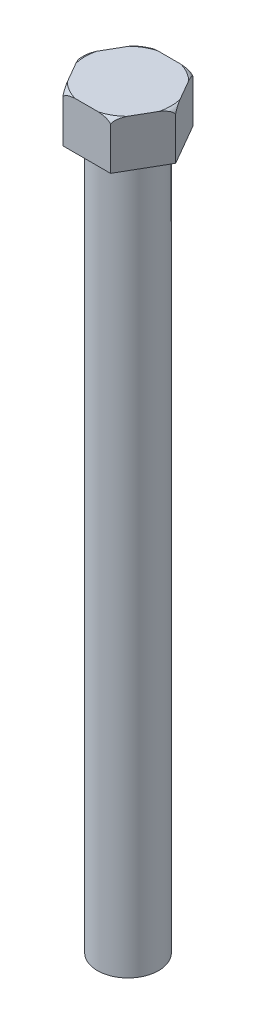
SolidWorks part; units mm, degrees
material "Plain Carbon Steel"
ref_plane "Front Plane" through (0, 0, 0) normal (0, 0, 1) x (1, 0, 0)
ref_plane "Top Plane" through (0, 0, 0) normal (0, 1, 0) x (1, 0, 0)
ref_plane "Right Plane" through (0, 0, 0) normal (1, 0, 0) x (0, 0, -1)
sketch "Hex Head Profile 35AF" plane through (0, 0, 0) normal (0, 1, 0) x (1, 0, 0)
  line L1 (20.2073, 0) -> (10.1036, 17.5)
  line L2 (10.1036, 17.5) -> (-10.1036, 17.5)
  line L3 (-10.1036, 17.5) -> (-20.2073, 0)
  line L4 (-20.2073, 0) -> (-10.1036, -17.5)
  line L5 (-10.1036, -17.5) -> (10.1036, -17.5)
  line L6 (10.1036, -17.5) -> (20.2073, 0)
  circle A0 centre (0, 0) radius 17.5 construction
  dimension "D1" = 35
extrude "Hex Head" add sketch "Hex Head Profile 35AF" along normal blind 20
sketch "Shank Profile Ø26" plane through (0, 0, 0) normal (0, -1, 0) x (1, 0, 0)
  circle A0 centre (0, 0) radius 13
  dimension "26" = 26
extrude "Shank Ø26x300" add sketch "Shank Profile Ø26" along normal blind 300
sketch "Head Chamfer Profile" plane through (0, 0, 0) normal (0, 0, 1) x (1, 0, 0)
  line L0 (10.1036, 20) -> (20.2073, 20) construction
  line L1 (20.2073, 20) -> (20.2073, 0) construction
  line L2 (18.2073, 20) -> (20.2073, 20)
  line L3 (20.2073, 20) -> (20.2073, 18)
  line L4 (0, 0) -> (0, 37.556) construction
  arc A0 (18.2073, 20) -> (20.2073, 18) centre (17.3364, 17.1292) cw
  dimension "D1" = 3
  dimension "D2" = 2
  dimension "D3" = 2
revolve "Head Chamfer" cut sketch "Head Chamfer Profile" angle 360 about L4
